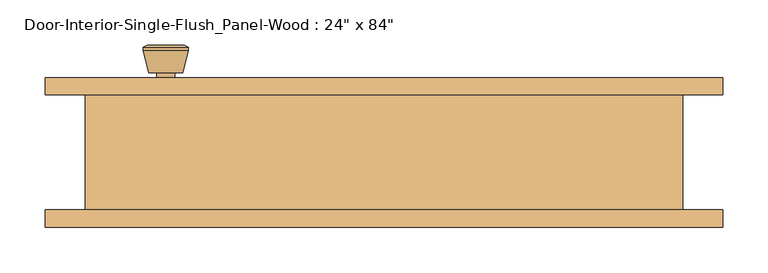
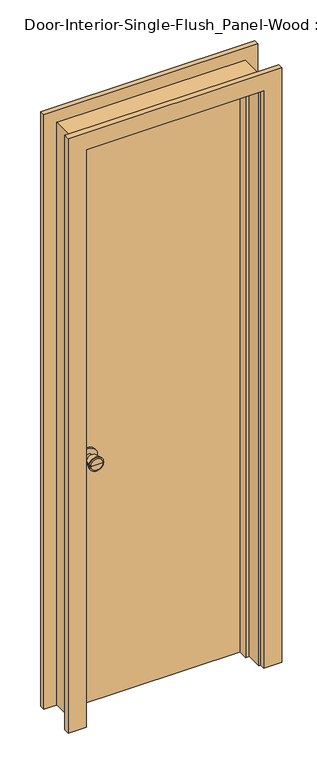
"""IFC4 building model written with IfcOpenShell, lengths in millimetres: door geometry."""

from ifc_helpers import new_model, si_unit, point, frame, frame_2d, origin, origin_with_axes, place, context, project, spatial, polyline, circle_curve, trimmed, segment, composite_curve, outline, extrude, faceted_brep, source, transform, mapped, element, save
from ifc_brep_helpers import plane_surface, cylinder_surface, revolved_surface, advanced_brep


def door_3f5f64ee(model_context):
    return source(origin(), model_context, "Body", "SolidModel", [
        advanced_brep(
        [(-241.3, 19.4, 914.4), (-231.3, 19.4, 914.4), (-251.3, 19.4, 914.4), (-220.8241324, -29.6, 914.4), (-241.3, -29.6, 914.4), (-261.7758676, -29.6, 914.4), (-216.3, -27.7721319, 914.4), (-266.3, -27.7721319, 914.4), (-216.3, -24.3084537, 914.4), (-266.3, -24.3084537, 914.4), (-222.663764, 0.4, 914.4), (-259.936236, 0.4, 914.4), (-231.3, 0.4, 914.4), (-251.3, 0.4, 914.4)],
        [
            (0, 1),
            (1, 2, circle_curve(frame((-241.3, 19.4, 914.4), z_axis=(0.0, 1.0, 0.0), x_axis=(-1.0, 0.0, 0.0)), 10.0)),
            (2, 0),
            (2, 1, circle_curve(frame((-241.3, 19.4, 914.4), z_axis=(0.0, 1.0, 0.0), x_axis=(-1.0, 0.0, 0.0)), 10.0)),
            (3, 4),
            (4, 5),
            (5, 3, circle_curve(frame((-241.3, -29.6, 914.4), z_axis=(0.0, -1.0, 0.0), x_axis=(-1.0, 0.0, 0.0)), 20.4758676)),
            (3, 5, circle_curve(frame((-241.3, -29.6, 914.4), z_axis=(0.0, -1.0, 0.0), x_axis=(-1.0, 0.0, 0.0)), 20.4758676)),
            (6, 3),
            (5, 7),
            (7, 6, circle_curve(frame((-241.3, -27.7721319, 914.4), z_axis=(0.0, -1.0, 0.0), x_axis=(-1.0, 0.0, 0.0)), 25.0)),
            (6, 7, circle_curve(frame((-241.3, -27.7721319, 914.4), z_axis=(0.0, -1.0, 0.0), x_axis=(-1.0, 0.0, 0.0)), 25.0)),
            (8, 6),
            (7, 9),
            (9, 8, circle_curve(frame((-241.3, -24.3084537, 914.4), z_axis=(0.0, -1.0, 0.0), x_axis=(-1.0, 0.0, 0.0)), 25.0)),
            (8, 9, circle_curve(frame((-241.3, -24.3084537, 914.4), z_axis=(0.0, -1.0, 0.0), x_axis=(-1.0, 0.0, 0.0)), 25.0)),
            (10, 8),
            (9, 11),
            (11, 10, circle_curve(frame((-241.3, 0.4, 914.4), z_axis=(0.0, -1.0, 0.0), x_axis=(-1.0, 0.0, 0.0)), 18.636236)),
            (10, 11, circle_curve(frame((-241.3, 0.4, 914.4), z_axis=(0.0, -1.0, 0.0), x_axis=(-1.0, 0.0, 0.0)), 18.636236)),
            (12, 10),
            (11, 13),
            (13, 12, circle_curve(frame((-241.3, 0.4, 914.4), z_axis=(0.0, -1.0, 0.0), x_axis=(-1.0, 0.0, 0.0)), 10.0)),
            (12, 13, circle_curve(frame((-241.3, 0.4, 914.4), z_axis=(0.0, -1.0, 0.0), x_axis=(-1.0, 0.0, 0.0)), 10.0)),
            (1, 12),
            (13, 2),
        ],
        [
            plane_surface(frame((-241.3, 19.4, 914.4), z_axis=(0.0, 1.0, 0.0), x_axis=(-1.0, 0.0, 0.0))),
            plane_surface(frame((-241.3, -29.6, 914.4), z_axis=(0.0, -1.0, 0.0), x_axis=(-1.0, 0.0, 0.0))),
            revolved_surface(polyline([(-261.7758676, -29.6, 914.4), (-266.3, -27.7721319, 914.4)]), (-241.3, 19.4, 914.4), (0.0, 1.0, 0.0)),
            cylinder_surface(frame((-241.3, 19.4, 914.4), z_axis=(0.0, 1.0, 0.0), x_axis=(-1.0, 0.0, 0.0)), 25.0),
            revolved_surface(polyline([(-266.3, -24.3084537, 914.4), (-259.936236, 0.4, 914.4)]), (-241.3, 19.4, 914.4), (0.0, 1.0, 0.0)),
            plane_surface(frame((-241.3, 0.4, 914.4), z_axis=(0.0, 1.0, 0.0), x_axis=(-1.0, 0.0, 0.0))),
            cylinder_surface(frame((-241.3, 19.4, 914.4), z_axis=(0.0, 1.0, 0.0), x_axis=(-1.0, 0.0, 0.0)), 10.0),
        ],
        [
            (0, [[1, 2, 3]]),
            (0, [[-3, 4, -1]]),
            (1, [[5, 6, 7]]),
            (1, [[-6, -5, 8]]),
            (2, [[9, -7, 10, 11]]),
            (2, [[-10, -8, -9, 12]]),
            (3, [[13, -11, 14, 15]]),
            (3, [[-14, -12, -13, 16]]),
            (4, [[17, -15, 18, 19]]),
            (4, [[-18, -16, -17, 20]]),
            (5, [[21, -19, 22, 23]]),
            (5, [[-22, -20, -21, 24]]),
            (6, [[25, -23, 26, -2]]),
            (6, [[-26, -24, -25, -4]]),
        ],
    ),
        extrude(outline(composite_curve([segment(trimmed(circle_curve(frame_2d((914.4, -241.3)), 30.0), [point((914.4, -271.3))], [point((914.4, -211.3))], False, "CARTESIAN"), True, "CONTINUOUS"), segment(trimmed(circle_curve(frame_2d((914.4, -241.3)), 30.0), [point((914.4, -211.3))], [point((914.4, -271.3))], False, "CARTESIAN"), True, "CONTINUOUS")], self_intersect=False)), frame((0.0, 19.4, 0.0), z_axis=(0.0, 1.0, 0.0), x_axis=(0.0, 0.0, 1.0)), (0.0, 0.0, 1.0), 6.0),
        advanced_brep(
        [(-241.3, 66.325, 914.4), (-251.3, 66.325, 914.4), (-231.3, 66.325, 914.4), (-220.8241324, 115.325, 914.4), (-261.7758676, 115.325, 914.4), (-241.3, 115.325, 914.4), (-216.3, 113.4971319, 914.4), (-266.3, 113.4971319, 914.4), (-216.3, 110.0334537, 914.4), (-266.3, 110.0334537, 914.4), (-222.663764, 85.325, 914.4), (-259.936236, 85.325, 914.4), (-231.3, 85.325, 914.4), (-251.3, 85.325, 914.4)],
        [
            (0, 1),
            (1, 2, circle_curve(frame((-241.3, 66.325, 914.4), z_axis=(0.0, -1.0, 0.0), x_axis=(-1.0, 0.0, 0.0)), 10.0)),
            (2, 0),
            (2, 1, circle_curve(frame((-241.3, 66.325, 914.4), z_axis=(0.0, -1.0, 0.0), x_axis=(-1.0, 0.0, 0.0)), 10.0)),
            (3, 4, circle_curve(frame((-241.3, 115.325, 914.4), z_axis=(0.0, 1.0, 0.0), x_axis=(-1.0, 0.0, 0.0)), 20.4758676)),
            (4, 5),
            (5, 3),
            (4, 3, circle_curve(frame((-241.3, 115.325, 914.4), z_axis=(0.0, 1.0, 0.0), x_axis=(-1.0, 0.0, 0.0)), 20.4758676)),
            (6, 7, circle_curve(frame((-241.3, 113.4971319, 914.4), z_axis=(0.0, 1.0, 0.0), x_axis=(-1.0, 0.0, 0.0)), 25.0)),
            (7, 4),
            (3, 6),
            (7, 6, circle_curve(frame((-241.3, 113.4971319, 914.4), z_axis=(0.0, 1.0, 0.0), x_axis=(-1.0, 0.0, 0.0)), 25.0)),
            (8, 9, circle_curve(frame((-241.3, 110.0334537, 914.4), z_axis=(0.0, 1.0, 0.0), x_axis=(-1.0, 0.0, 0.0)), 25.0)),
            (9, 7),
            (6, 8),
            (9, 8, circle_curve(frame((-241.3, 110.0334537, 914.4), z_axis=(0.0, 1.0, 0.0), x_axis=(-1.0, 0.0, 0.0)), 25.0)),
            (10, 11, circle_curve(frame((-241.3, 85.325, 914.4), z_axis=(0.0, 1.0, 0.0), x_axis=(-1.0, 0.0, 0.0)), 18.636236)),
            (11, 9),
            (8, 10),
            (11, 10, circle_curve(frame((-241.3, 85.325, 914.4), z_axis=(0.0, 1.0, 0.0), x_axis=(-1.0, 0.0, 0.0)), 18.636236)),
            (12, 13, circle_curve(frame((-241.3, 85.325, 914.4), z_axis=(0.0, 1.0, 0.0), x_axis=(-1.0, 0.0, 0.0)), 10.0)),
            (13, 11),
            (10, 12),
            (13, 12, circle_curve(frame((-241.3, 85.325, 914.4), z_axis=(0.0, 1.0, 0.0), x_axis=(-1.0, 0.0, 0.0)), 10.0)),
            (1, 13),
            (12, 2),
        ],
        [
            plane_surface(frame((-241.3, 66.325, 914.4), z_axis=(0.0, -1.0, 0.0), x_axis=(-1.0, 0.0, 0.0))),
            plane_surface(frame((-241.3, 115.325, 914.4), z_axis=(0.0, 1.0, 0.0), x_axis=(-1.0, 0.0, 0.0))),
            revolved_surface(polyline([(-261.7758676, 115.325, 914.4), (-266.3, 113.4971319, 914.4)]), (-241.3, 66.325, 914.4), (0.0, -1.0, 0.0)),
            cylinder_surface(frame((-241.3, 66.325, 914.4), z_axis=(0.0, -1.0, 0.0), x_axis=(-1.0, 0.0, 0.0)), 25.0),
            revolved_surface(polyline([(-266.3, 110.0334537, 914.4), (-259.936236, 85.325, 914.4)]), (-241.3, 66.325, 914.4), (0.0, -1.0, 0.0)),
            plane_surface(frame((-241.3, 85.325, 914.4), z_axis=(0.0, -1.0, 0.0), x_axis=(-1.0, 0.0, 0.0))),
            cylinder_surface(frame((-241.3, 66.325, 914.4), z_axis=(0.0, -1.0, 0.0), x_axis=(-1.0, 0.0, 0.0)), 10.0),
        ],
        [
            (0, [[1, 2, 3]]),
            (0, [[-3, 4, -1]]),
            (1, [[5, 6, 7]]),
            (1, [[8, -7, -6]]),
            (2, [[9, 10, -5, 11]]),
            (2, [[12, -11, -8, -10]]),
            (3, [[13, 14, -9, 15]]),
            (3, [[16, -15, -12, -14]]),
            (4, [[17, 18, -13, 19]]),
            (4, [[20, -19, -16, -18]]),
            (5, [[21, 22, -17, 23]]),
            (5, [[24, -23, -20, -22]]),
            (6, [[-2, 25, -21, 26]]),
            (6, [[-4, -26, -24, -25]]),
        ],
    ),
        extrude(outline(composite_curve([segment(trimmed(circle_curve(frame_2d((914.4, -241.3)), 30.0), [point((914.4, -271.3))], [point((914.4, -211.3))], False, "CARTESIAN"), True, "CONTINUOUS"), segment(trimmed(circle_curve(frame_2d((914.4, -241.3)), 30.0), [point((914.4, -211.3))], [point((914.4, -271.3))], False, "CARTESIAN"), True, "CONTINUOUS")], self_intersect=False)), frame((0.0, 60.325, 0.0), z_axis=(0.0, 1.0, 0.0), x_axis=(0.0, 0.0, 1.0)), (0.0, 0.0, 1.0), 6.0),
        faceted_brep([(330.2, 60.325, 0.0), (330.2, -66.675, 0.0), (304.8, -66.675, 0.0), (304.8, -9.525, 0.0), (292.1, -9.525, 0.0), (292.1, 25.4, 0.0), (304.8, 25.4, 0.0), (304.8, 60.325, 0.0), (330.2, 60.325, 2159.0), (330.2, -66.675, 2159.0), (-330.2, -66.675, 2159.0), (-330.2, -66.675, 0.0), (-304.8, -66.675, 0.0), (-304.8, -66.675, 2133.6), (304.8, -66.675, 2133.6), (304.8, -9.525, 2133.6), (-304.8, -9.525, 2133.6), (-304.8, -9.525, 0.0), (-292.1, -9.525, 0.0), (-292.1, -9.525, 2120.9), (292.1, -9.525, 2120.9), (292.1, 25.4, 2120.9), (-292.1, 25.4, 2120.9), (-292.1, 25.4, 0.0), (-304.8, 25.4, 0.0), (-304.8, 25.4, 2133.6), (304.8, 25.4, 2133.6), (304.8, 60.325, 2133.6), (-304.8, 60.325, 2133.6), (-304.8, 60.325, 0.0), (-330.2, 60.325, 0.0), (-330.2, 60.325, 2159.0)], [[[0, 1, 2, 3, 4, 5, 6, 7]], [[1, 0, 8, 9]], [[2, 1, 9, 10, 11, 12, 13, 14]], [[3, 2, 14, 15]], [[4, 3, 15, 16, 17, 18, 19, 20]], [[5, 4, 20, 21]], [[6, 5, 21, 22, 23, 24, 25, 26]], [[7, 6, 26, 27]], [[0, 7, 27, 28, 29, 30, 31, 8]], [[9, 8, 31, 10]], [[15, 14, 13, 16]], [[21, 20, 19, 22]], [[27, 26, 25, 28]], [[30, 29, 24, 23, 18, 17, 12, 11]], [[10, 31, 30, 11]], [[16, 13, 12, 17]], [[22, 19, 18, 23]], [[28, 25, 24, 29]]]),
        extrude(outline(polyline([(304.8, 25.4), (-304.8, 25.4), (-304.8, 60.325), (304.8, 60.325), (304.8, 25.4)])), origin_with_axes(), (0.0, 0.0, 1.0), 2133.6),
        extrude(outline(polyline([(0.0, 311.15), (0.0, 374.65), (2203.45, 374.65), (2203.45, -374.65), (0.0, -374.65), (0.0, -311.15), (2139.95, -311.15), (2139.95, 311.15), (0.0, 311.15)])), frame((0.0, 60.325, 0.0), z_axis=(0.0, 1.0, 0.0), x_axis=(0.0, 0.0, 1.0)), (0.0, 0.0, 1.0), 19.05),
        extrude(outline(polyline([(0.0, 311.15), (0.0, 374.65), (2203.45, 374.65), (2203.45, -374.65), (0.0, -374.65), (0.0, -311.15), (2139.95, -311.15), (2139.95, 311.15), (0.0, 311.15)])), frame((0.0, -85.725, 0.0), z_axis=(0.0, 1.0, 0.0), x_axis=(0.0, 0.0, 1.0)), (0.0, 0.0, 1.0), 19.05),
    ])


if __name__ == "__main__":
    model = new_model("IFC4")
    model_context = context("Model", 3, world=origin())
    ifc_project = project(units=[si_unit("LENGTHUNIT", "METRE", prefix="MILLI")], contexts=[model_context])
    site = spatial("IfcSite", under=ifc_project)
    building = spatial("IfcBuilding", under=site)
    placement = place(None, origin())
    door_shape = door_3f5f64ee(model_context)
    element("IfcDoor", 1, ObjectType="Door-Interior-Single-Flush_Panel-Wood : 24\" x 84\"", at=placement, inside=building, context=model_context, shape_type="MappedRepresentation", body=[
        mapped(door_shape, transform((0.0, 0.0, 0.0), x_axis=(1.0, 0.0, 0.0), y_axis=(0.0, 1.0, 0.0), z_axis=(0.0, 0.0, 1.0))),
    ])
    save(model, "model.ifc")

# Revit data of these elements
# Type "Door-Interior-Single-Flush_Panel-Wood : 24\" x 84\""
#   Type Mark = "11"
#   Assembly Code = "C1020300"
#   Analytic Construction = "Wooden"
#   Thickness = 0' - 1 3/8"
#   Thermal Resistance (R) = 2.5876 (h·ft²·°F)/BTU
#   Swing Angle [instance default] = 90.00°
#   Rough Width = 2' - 2"
#   Rough Height = 7' - 1"
#   Height = 7' - 0"
#   Width = 2' - 0"
#   Heat Transfer Coefficient (U) = 0.3865 BTU/(h·ft²·°F)
#   Trim Material = Cherry
#   Panel Material = Cherry
#   Frame Material = Cherry
#   Door Handle Material = Aluminum
#   Visual Light Transmittance = 0
#   Solar Heat Gain Coefficient = 0
#   Wall Closure = (empty or 0)
#   Function = (empty or 0)
# Element 1 (IfcDoor, "Door-Interior-Single-Flush_Panel-Wood : 24\" x 84\"")
#   Materials on its faces: "Cherry", "Aluminum"
# Materials
#   "Cherry": class "Wood", colour RGB 226 177 128, transparency 0, Description = "Prunus Serotina", Cost = 0
#   "Aluminum": class "Metal", colour RGB 247 247 247, transparency 0, Description = "Aluminum 6061", Cost = 0
